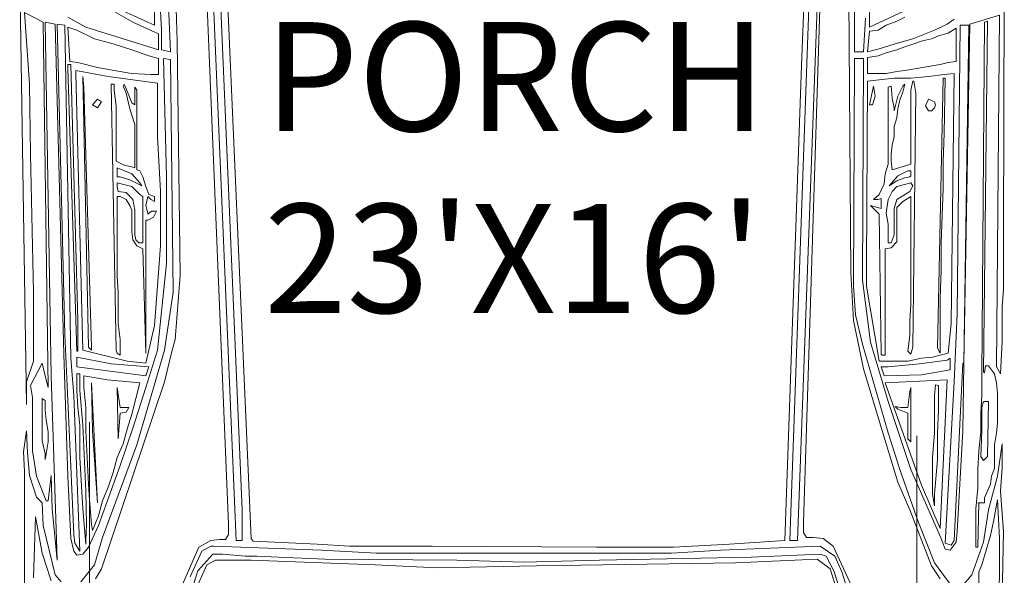
# Model space of a CAD drawing. Units: inches. Extents: x -9 to 646, y -802 to 47.
# Tile 5 of 17: x 432 to 486, y -633 to -602. Entities that reach past the tile are written whole.
import ezdxf

# ---------------------------------------------------------------- set-up
doc = ezdxf.new("R2010")
doc.units = ezdxf.units.IN
doc.header["$MEASUREMENT"] = 0
doc.layers.add('A-AREA-IDEN', color=7, linetype='Continuous', lineweight=18)
doc.layers.add('A-SITE-VEHI', color=8, linetype='Continuous', lineweight=9)
doc.styles.get("Standard").update_dxf_attribs({"font": 'arial.ttf'})

msp = doc.modelspace()

# ---------------------------------------------------------------- linework, layer by layer
at = {"layer": 'A-SITE-VEHI'}
for p, q in [((439.87, -602.535), (439.275, -591.315)), ((439.87, -591.424), (440.358, -603.727)), ((440.467, -594.892), (440.738, -603.132)), ((475.643, -597.277), (474.451, -630.612)), ((478.894, -596.79), (478.841, -602.373)), ((475.102, -604.487), (475.372, -597.821)), ((478.028, -603.727), (478.028, -597.765)), ((443.394, -598.092), (444.801, -630.503)), ((474.884, -630.612), (476.076, -598.254)), ((432.065, -599.608), (432.445, -623.132)), ((486.213, -613.808), (486.266, -599.77)), ((438.298, -602.102), (434.721, -600.041)), ((443.556, -629.744), (442.363, -600.53)), ((475.208, -629.635), (476.13, -600.476)), ((477.702, -600.312), (477.811, -615.869)), ((444.315, -628.931), (443.123, -600.909)), ((432.607, -605.517), (432.336, -601.56)), ((432.336, -601.56), (433.366, -602.102)), ((437.214, -601.234), (439.49, -602.264)), ((439.49, -602.264), (439.49, -601.398)), ((442.743, -601.505), (443.989, -630.612)), ((478.841, -602.373), (481.279, -601.234)), ((433.366, -602.102), (433.637, -622.21)), ((433.799, -621.56), (433.475, -602.102)), ((433.475, -602.102), (434.017, -602.211)), ((434.721, -601.831), (435.698, -602.373)), ((439.708, -602.752), (438.298, -602.102)), ((478.623, -601.884), (478.514, -603.727)), ((479.762, -602.264), (480.357, -602.048)), ((480.357, -602.048), (480.793, -601.831)), ((483.502, -601.94), (483.122, -602.211)), ((484.37, -602.211), (485.995, -601.722)), ((485.182, -602.102), (485.02, -621.56)), ((485.127, -621.342), (485.345, -602.048)), ((485.345, -602.048), (485.182, -602.102)), ((485.995, -601.722), (485.833, -621.071)), ((434.017, -602.211), (434.503, -620.367)), ((434.558, -602.264), (434.125, -602.211)), ((434.125, -602.211), (434.558, -619.284)), ((434.883, -620.585), (434.558, -602.264)), ((435.209, -602.535), (434.721, -602.373)), ((434.721, -602.373), (434.829, -604.269)), ((436.184, -603.023), (435.209, -602.535)), ((435.698, -602.373), (439.708, -603.618)), ((439.87, -603.618), (439.87, -602.535)), ((478.732, -603.727), (478.841, -602.59)), ((478.841, -602.59), (479.329, -602.535)), ((479.329, -602.535), (479.762, -602.264)), ((482.418, -602.535), (481.226, -603.023)), ((483.122, -602.211), (482.418, -602.535)), ((483.177, -602.697), (482.636, -602.861)), ((483.61, -602.426), (483.177, -602.697)), ((483.61, -604.269), (483.61, -602.426)), ((483.664, -618.145), (483.828, -602.264)), ((483.828, -602.264), (484.314, -602.264)), ((484.043, -620.856), (484.37, -602.211)), ((484.314, -602.264), (484.043, -620.856)), ((437.214, -603.294), (436.184, -603.023)), ((439.708, -603.618), (439.708, -602.752)), ((440.738, -603.132), (440.9, -616.031)), ((481.226, -603.023), (480.251, -603.294)), ((481.767, -603.132), (481.279, -603.294)), ((482.256, -603.023), (481.767, -603.132)), ((482.636, -602.861), (482.256, -603.023)), ((438.244, -603.618), (437.214, -603.294)), ((439.166, -603.945), (438.244, -603.618)), ((440.358, -603.727), (439.87, -603.618)), ((478.514, -603.727), (478.028, -603.727)), ((479.383, -603.565), (478.732, -603.727)), ((479.762, -603.783), (479.329, -603.945)), ((480.251, -603.294), (479.383, -603.565)), ((480.357, -603.618), (479.762, -603.783)), ((480.793, -603.456), (480.357, -603.618)), ((481.279, -603.294), (480.793, -603.456)), ((434.829, -604.269), (435.262, -604.324)), ((435.262, -604.324), (436.346, -604.595)), ((439.708, -604.107), (439.166, -603.945)), ((439.708, -604.975), (439.708, -604.107)), ((440.141, -610.611), (439.979, -604.107)), ((439.979, -604.107), (440.358, -604.162)), ((440.358, -604.162), (440.52, -616.952)), ((477.973, -616.628), (478.028, -604.107)), ((478.028, -604.107), (478.514, -604.107)), ((478.514, -604.107), (478.461, -616.302)), ((479.329, -603.945), (478.732, -604.054)), ((478.732, -604.054), (478.732, -604.92)), ((482.742, -604.433), (483.177, -604.324)), ((483.177, -604.324), (483.61, -604.269)), ((434.883, -604.433), (434.721, -604.433)), ((434.721, -604.433), (434.721, -604.649)), ((434.721, -604.649), (435.209, -620.205)), ((435.262, -618.524), (434.883, -604.433)), ((436.943, -605.082), (435.154, -604.757)), ((435.154, -604.757), (435.154, -604.92)), ((436.346, -604.595), (437.267, -604.757)), ((437.267, -604.757), (438.244, -604.92)), ((474.18, -630.612), (475.102, -604.487)), ((479.762, -604.92), (480.357, -604.811)), ((480.357, -604.811), (480.793, -604.757)), ((480.793, -604.757), (482.742, -604.433)), ((435.154, -604.92), (435.533, -620.15)), ((435.589, -605.679), (435.533, -605.082)), ((435.533, -605.082), (435.86, -619.987)), ((439.652, -605.461), (436.943, -605.082)), ((438.244, -604.92), (439.275, -604.975)), ((439.275, -604.975), (439.708, -604.975)), ((478.732, -605.355), (478.679, -615.544)), ((478.732, -604.92), (479.762, -604.92)), ((479.221, -605.299), (478.732, -605.355)), ((480.195, -605.19), (479.221, -605.299)), ((481.117, -605.19), (480.195, -605.19)), ((482.092, -605.082), (481.117, -605.19)), ((481.226, -605.355), (481.117, -605.841)), ((481.279, -605.355), (481.226, -605.355)), ((481.388, -606.003), (481.279, -605.355)), ((482.96, -604.975), (482.092, -605.082)), ((482.906, -605.19), (482.742, -613.051)), ((483.013, -605.19), (482.906, -605.19)), ((483.502, -604.92), (482.96, -604.975)), ((482.96, -608.226), (483.013, -605.19)), ((483.339, -618.686), (483.502, -604.92)), ((432.662, -609.365), (432.607, -605.517)), ((436.022, -619.987), (435.589, -605.679)), ((437.267, -605.517), (437.105, -605.517)), ((437.105, -605.517), (437.376, -620.15)), ((437.267, -605.841), (437.267, -605.517)), ((437.376, -606.709), (437.267, -605.841)), ((437.811, -605.517), (437.756, -605.626)), ((437.756, -605.626), (437.918, -606.003)), ((438.082, -606.112), (437.811, -605.517)), ((438.515, -605.841), (438.407, -605.679)), ((438.407, -605.679), (438.407, -606.654)), ((438.515, -610.231), (438.515, -605.841)), ((439.652, -608.388), (439.652, -605.461)), ((479.058, -605.626), (478.841, -606.654)), ((479.165, -606.167), (479.058, -605.626)), ((480.033, -605.626), (479.871, -605.679)), ((479.871, -605.679), (479.871, -609.907)), ((480.087, -606.276), (480.033, -605.626)), ((480.684, -605.626), (480.413, -606.167)), ((480.522, -606.383), (480.684, -605.95)), ((480.684, -605.95), (480.793, -605.517)), ((480.793, -605.517), (480.684, -605.626)), ((481.117, -605.841), (481.117, -609.907)), ((436.346, -606.329), (436.075, -606.654)), ((436.564, -606.492), (436.346, -606.329)), ((436.346, -606.818), (436.564, -606.492)), ((437.918, -606.003), (438.136, -606.871)), ((438.244, -606.547), (438.082, -606.112)), ((479.003, -606.654), (479.058, -606.492)), ((479.058, -606.492), (479.165, -606.167)), ((480.195, -606.818), (480.087, -606.276)), ((480.413, -606.167), (480.195, -606.98)), ((480.413, -606.871), (480.522, -606.383)), ((481.226, -619.987), (481.388, -606.003)), ((482.092, -606.329), (481.93, -606.709)), ((482.418, -606.492), (482.092, -606.329)), ((482.471, -606.654), (482.418, -606.492)), ((436.075, -606.654), (436.346, -606.818)), ((437.376, -609.745), (437.376, -606.709)), ((438.136, -606.871), (438.407, -607.739)), ((438.407, -606.654), (438.244, -606.547)), ((478.841, -606.654), (479.003, -606.654)), ((480.195, -606.98), (480.195, -606.818)), ((480.357, -607.36), (480.413, -606.871)), ((481.93, -606.709), (482.092, -606.98)), ((482.092, -606.98), (482.256, -606.98)), ((482.256, -606.98), (482.418, -606.818)), ((482.418, -606.818), (482.471, -606.654)), ((480.195, -607.846), (480.357, -607.36)), ((438.407, -607.739), (438.407, -610.124)), ((480.195, -608.388), (480.195, -607.846)), ((439.816, -611.423), (439.652, -608.388)), ((480.087, -608.876), (480.195, -608.388)), ((482.906, -609.745), (482.96, -608.226)), ((480.033, -609.365), (480.087, -608.876)), ((432.824, -616.952), (432.662, -609.365)), ((437.811, -609.96), (437.376, -609.745)), ((480.033, -609.745), (480.033, -609.365)), ((480.087, -610.231), (480.033, -609.745)), ((482.906, -611.261), (482.906, -609.745)), ((438.244, -610.448), (437.432, -610.124)), ((437.432, -610.124), (437.432, -610.611)), ((438.244, -610.069), (437.811, -609.96)), ((438.407, -610.124), (438.244, -610.069)), ((438.677, -610.286), (438.515, -610.231)), ((438.84, -610.611), (438.677, -610.286)), ((479.871, -609.907), (479.707, -610.448)), ((481.117, -609.907), (480.087, -610.231)), ((480.955, -610.286), (480.413, -610.557)), ((481.117, -610.286), (480.955, -610.286)), ((481.117, -610.557), (481.117, -610.286)), ((437.432, -610.611), (437.594, -610.611)), ((437.594, -610.611), (438.136, -610.775)), ((438.136, -610.775), (438.786, -611.099)), ((438.677, -610.937), (438.244, -610.448)), ((439.004, -611.152), (438.84, -610.611)), ((440.141, -615.38), (440.141, -610.611)), ((479.707, -610.448), (479.654, -610.99)), ((480.413, -610.557), (479.924, -611.099)), ((479.924, -611.099), (480.357, -610.828)), ((480.357, -610.828), (480.793, -610.666)), ((480.793, -610.666), (481.064, -610.611)), ((481.064, -610.611), (481.117, -610.557)), ((438.244, -611.152), (437.432, -610.937)), ((437.432, -610.937), (437.432, -611.152)), ((437.432, -611.152), (437.485, -611.423)), ((438.677, -611.587), (438.244, -611.152)), ((438.786, -611.099), (438.677, -610.937)), ((439.166, -611.587), (439.004, -611.152)), ((479.654, -610.99), (479.383, -611.587)), ((480.357, -611.152), (480.087, -611.423)), ((481.117, -610.937), (480.357, -611.152)), ((481.064, -611.423), (481.226, -611.099)), ((481.226, -611.099), (481.117, -610.937)), ((482.798, -614.243), (482.906, -611.261)), ((437.432, -616.086), (437.432, -611.696)), ((437.432, -611.696), (437.594, -611.696)), ((437.485, -611.423), (437.918, -611.479)), ((437.594, -611.696), (437.918, -611.858)), ((437.918, -611.479), (438.298, -611.858)), ((437.918, -611.858), (438.136, -612.183)), ((438.298, -611.858), (438.407, -612.454)), ((438.84, -611.696), (438.677, -611.587)), ((438.84, -614.243), (438.84, -611.696)), ((439.004, -612.183), (439.11, -611.696)), ((439.11, -611.696), (439.275, -611.858)), ((439.49, -611.696), (439.166, -611.587)), ((439.275, -611.858), (439.49, -611.967)), ((439.49, -611.967), (439.49, -611.696)), ((439.816, -614.405), (439.816, -611.423)), ((479.383, -611.587), (479.058, -611.858)), ((479.058, -611.858), (479.329, -611.858)), ((479.329, -611.858), (479.491, -611.803)), ((479.491, -611.803), (479.491, -612.345)), ((479.871, -611.858), (479.762, -612.616)), ((480.087, -611.423), (479.871, -611.858)), ((480.195, -612.345), (480.357, -611.858)), ((480.357, -611.858), (481.064, -611.423)), ((480.684, -611.967), (481.117, -611.696)), ((481.117, -611.696), (481.117, -617.658)), ((438.136, -612.183), (438.244, -612.454)), ((438.244, -612.454), (438.244, -613.646)), ((438.407, -612.454), (438.407, -613.808)), ((439.11, -612.616), (439.004, -612.183)), ((479.491, -612.345), (478.894, -612.183)), ((478.894, -612.183), (479.383, -612.671)), ((480.195, -613.808), (480.195, -612.345)), ((480.357, -612.291), (480.684, -611.967)), ((480.357, -614.188), (480.357, -612.291)), ((439.004, -620.314), (439.004, -612.995)), ((439.004, -612.995), (439.11, -612.995)), ((439.328, -612.509), (439.11, -612.671)), ((439.11, -612.671), (439.11, -612.616)), ((439.11, -612.995), (439.437, -612.833)), ((439.599, -612.509), (439.328, -612.509)), ((439.437, -612.833), (439.599, -612.509)), ((479.383, -612.671), (479.491, -620.367)), ((479.762, -612.616), (479.871, -613.213)), ((479.871, -613.213), (479.871, -614.243)), ((482.742, -613.051), (482.58, -620.043)), ((438.244, -613.646), (438.298, -614.081)), ((438.298, -614.081), (438.515, -614.405)), ((438.407, -613.808), (438.46, -614.081)), ((438.46, -614.081), (438.624, -614.243)), ((480.033, -614.243), (480.195, -613.808)), ((486.213, -616.79), (486.213, -613.808)), ((438.515, -614.405), (438.84, -614.567)), ((438.624, -614.243), (438.84, -614.243)), ((438.84, -614.567), (439.004, -620.314)), ((439.49, -618.795), (439.816, -614.405)), ((479.707, -614.567), (480.033, -614.514)), ((479.707, -620.423), (479.707, -614.567)), ((479.871, -614.243), (480.033, -614.243)), ((480.033, -614.514), (480.357, -614.188)), ((482.798, -615.76), (482.798, -614.243)), ((439.652, -620.15), (440.141, -615.38)), ((478.679, -615.544), (478.679, -616.628)), ((437.485, -616.952), (437.432, -616.086)), ((440.9, -616.031), (440.629, -619.554)), ((477.811, -615.869), (477.973, -618.524)), ((482.742, -617.278), (482.798, -615.76)), ((478.081, -618.2), (477.973, -616.628)), ((478.461, -616.302), (478.894, -619.717)), ((478.679, -616.628), (479.383, -620.747)), ((486.157, -617.765), (486.213, -616.79)), ((432.824, -620.747), (432.824, -616.952)), ((437.485, -618.686), (437.485, -616.952)), ((440.52, -616.952), (440.032, -620.15)), ((482.742, -620.314), (482.742, -617.278)), ((481.117, -617.658), (481.064, -618.524)), ((486.157, -619.663), (486.157, -617.765)), ((478.461, -619.825), (478.081, -618.2)), ((483.502, -621.886), (483.664, -618.145)), ((435.262, -620.205), (435.262, -618.524)), ((437.594, -619.554), (437.485, -618.686)), ((439.004, -620.856), (439.49, -618.795)), ((477.973, -618.524), (478.514, -621.18)), ((481.064, -618.524), (481.064, -619.337)), ((483.177, -620.314), (483.339, -618.686)), ((434.558, -619.284), (434.883, -626.547)), ((481.064, -619.337), (480.955, -620.205)), ((435.86, -619.987), (436.022, -620.15)), ((436.022, -620.15), (436.022, -619.987)), ((437.594, -620.423), (437.594, -619.554)), ((440.629, -619.554), (440.467, -620.15)), ((479.871, -624.704), (478.461, -619.825)), ((478.894, -619.717), (479.871, -622.97)), ((481.117, -620.367), (481.226, -619.987)), ((482.58, -620.043), (482.742, -620.314)), ((486.048, -621.451), (486.157, -619.663)), ((434.503, -620.367), (434.721, -627.088)), ((435.047, -622.643), (434.883, -620.585)), ((435.209, -620.205), (435.262, -620.205)), ((437.105, -620.909), (435.209, -620.529)), ((435.209, -620.529), (435.209, -621.071)), ((435.533, -620.15), (437.974, -620.747)), ((437.376, -620.15), (437.432, -620.314)), ((437.432, -620.314), (437.594, -620.423)), ((440.032, -620.15), (438.515, -625.354)), ((439.004, -622.21), (439.652, -620.15)), ((440.467, -620.15), (440.032, -621.886)), ((479.491, -620.367), (479.545, -620.423)), ((479.545, -620.423), (479.707, -620.423)), ((480.955, -620.205), (481.117, -620.367)), ((480.955, -620.747), (481.714, -620.585)), ((481.714, -620.585), (482.309, -620.529)), ((482.309, -620.529), (482.742, -620.423)), ((482.742, -620.423), (483.177, -620.314)), ((483.284, -620.585), (483.122, -620.694)), ((483.284, -621.235), (483.284, -620.585)), ((432.445, -621.886), (432.824, -620.747)), ((433.311, -620.856), (432.662, -622.101)), ((433.475, -621.56), (433.311, -620.856)), ((435.209, -621.071), (439.004, -621.56)), ((439.166, -621.071), (437.105, -620.909)), ((437.974, -620.747), (439.004, -620.856)), ((439.004, -621.56), (439.166, -621.071)), ((479.383, -620.747), (480.955, -620.747)), ((479.871, -621.071), (479.491, -621.071)), ((479.491, -621.071), (479.654, -621.56)), ((481.605, -620.909), (479.871, -621.071)), ((483.122, -620.694), (481.605, -620.909)), ((483.99, -620.856), (483.502, -630.612)), ((484.043, -620.856), (483.99, -620.856)), ((483.99, -624.595), (484.043, -620.909)), ((484.043, -620.909), (484.043, -620.856)), ((485.236, -621.018), (485.182, -621.397)), ((485.398, -621.018), (485.236, -621.018)), ((485.724, -621.451), (485.398, -621.018)), ((485.833, -621.071), (486.048, -621.451)), ((433.637, -622.21), (433.475, -621.56)), ((434.125, -631.696), (433.799, -621.56)), ((435.371, -621.451), (435.209, -621.451)), ((435.209, -621.451), (435.209, -622.372)), ((435.371, -622.372), (435.371, -621.451)), ((436.89, -621.777), (435.589, -621.56)), ((435.589, -621.56), (435.589, -622.21)), ((478.514, -621.18), (479.762, -625.299)), ((479.654, -621.56), (481.714, -621.506)), ((481.714, -621.506), (483.284, -621.235)), ((485.02, -621.56), (485.02, -622.643)), ((485.182, -621.397), (485.127, -621.342)), ((485.833, -621.939), (485.724, -621.451)), ((432.445, -623.132), (432.445, -621.886)), ((432.662, -622.101), (432.769, -622.752)), ((435.589, -622.21), (435.698, -623.294)), ((436.346, -628.552), (436.022, -621.939)), ((436.022, -621.939), (436.075, -624.595)), ((440.032, -621.886), (436.564, -632.182)), ((438.677, -621.939), (436.89, -621.777)), ((437.594, -623.294), (437.432, -622.21)), ((437.432, -622.21), (437.485, -625.028)), ((438.298, -624.433), (439.004, -622.21)), ((438.46, -622.807), (438.677, -621.939)), ((483.122, -621.777), (479.707, -621.939)), ((479.707, -621.939), (481.714, -627.577)), ((481.117, -622.21), (481.064, -622.428)), ((481.117, -625.192), (481.117, -622.21)), ((482.471, -622.048), (482.418, -622.643)), ((482.636, -622.101), (482.471, -622.048)), ((482.636, -623.456), (482.636, -622.101)), ((482.742, -629.962), (483.122, -621.777)), ((483.013, -630.774), (483.502, -621.886)), ((485.886, -622.536), (485.833, -621.939)), ((432.769, -622.752), (432.769, -625.678)), ((435.371, -631.207), (435.047, -622.643)), ((435.209, -622.372), (435.262, -623.294)), ((435.533, -624.271), (435.371, -622.372)), ((481.064, -622.428), (480.955, -623.294)), ((482.418, -622.643), (482.418, -624.704)), ((485.02, -622.643), (484.965, -623.62)), ((485.886, -624.162), (485.886, -622.536)), ((433.475, -622.914), (433.311, -622.807)), ((433.311, -622.807), (433.311, -625.137)), ((433.475, -623.456), (433.475, -622.914)), ((435.262, -623.294), (435.371, -624.271)), ((435.698, -623.294), (435.698, -624.595)), ((438.082, -623.294), (437.594, -623.294)), ((437.918, -623.565), (438.082, -623.294)), ((438.244, -623.673), (438.46, -622.807)), ((479.871, -622.97), (481.117, -626.709)), ((480.575, -623.294), (480.251, -623.24)), ((480.251, -623.24), (480.413, -623.403)), ((480.955, -623.294), (480.575, -623.294)), ((485.127, -622.97), (485.02, -623.294)), ((485.02, -623.294), (485.02, -624.595)), ((485.398, -622.97), (485.127, -622.97)), ((485.345, -626.005), (485.398, -622.97)), ((433.528, -624), (433.475, -623.456)), ((437.485, -625.028), (437.594, -623.62)), ((437.594, -623.62), (437.918, -623.565)), ((437.974, -624.486), (438.244, -623.673)), ((480.413, -623.403), (480.955, -623.62)), ((480.955, -623.62), (480.955, -625.028)), ((482.58, -624.704), (482.636, -623.456)), ((484.965, -623.62), (484.965, -624.648)), ((433.637, -624.648), (433.528, -624)), ((435.371, -624.271), (435.371, -626.058)), ((435.698, -627.901), (435.533, -624.271)), ((435.913, -624.106), (435.913, -643.944)), ((485.833, -624.704), (485.886, -624.162)), ((432.445, -624.595), (432.283, -625.734)), ((432.498, -625.787), (432.445, -624.595)), ((433.637, -625.192), (433.637, -624.648)), ((435.698, -624.595), (435.86, -627.521)), ((436.075, -624.595), (436.346, -628.552)), ((437.594, -626.491), (438.298, -624.433)), ((437.756, -625.299), (437.974, -624.486)), ((480.522, -626.709), (479.871, -624.704)), ((481.443, -624.866), (481.443, -644.812)), ((482.418, -624.704), (482.309, -626.058)), ((482.58, -626.167), (482.58, -624.704)), ((483.664, -630.124), (483.99, -624.595)), ((484.965, -624.648), (484.856, -625.678)), ((485.02, -624.595), (484.965, -626.005)), ((485.724, -625.354), (485.833, -624.704)), ((433.311, -625.137), (433.475, -625.843)), ((433.528, -625.843), (433.637, -625.192)), ((438.515, -625.354), (436.617, -630.448)), ((437.432, -626.058), (437.756, -625.299)), ((479.762, -625.299), (480.413, -627.413)), ((480.955, -625.028), (481.117, -625.192)), ((485.724, -626.655), (485.724, -625.354)), ((486.157, -625.299), (485.886, -627.088)), ((486.157, -626.6), (486.157, -625.299)), ((432.283, -625.734), (432.336, -626.818)), ((432.607, -627.035), (432.498, -625.787)), ((432.769, -625.678), (432.986, -627.088)), ((433.475, -626.167), (433.528, -625.843)), ((433.475, -625.843), (433.475, -626.167)), ((484.856, -625.678), (484.803, -626.709)), ((484.965, -626.005), (485.127, -626.22)), ((485.127, -626.22), (485.345, -626.005)), ((434.883, -626.547), (435.047, -630.286)), ((435.371, -626.058), (435.533, -628.876)), ((436.401, -629.797), (437.594, -626.491)), ((437.214, -626.871), (437.432, -626.058)), ((482.309, -626.058), (482.309, -628.063)), ((482.418, -628.063), (482.58, -626.167)), ((432.336, -626.818), (432.336, -636.303)), ((432.986, -628.228), (432.607, -627.035)), ((432.986, -627.088), (433.528, -628.443)), ((433.637, -628.443), (433.799, -627.035)), ((433.799, -627.035), (433.855, -628.876)), ((434.721, -627.088), (434.883, -630.503)), ((436.943, -627.684), (437.214, -626.871)), ((481.55, -629.635), (480.522, -626.709)), ((481.117, -626.709), (482.798, -630.503)), ((484.803, -626.709), (484.803, -627.739)), ((485.886, -627.088), (485.398, -628.931)), ((485.507, -627.521), (485.562, -627.088)), ((485.562, -627.088), (485.724, -626.655)), ((486.048, -627.901), (486.157, -626.6)), ((435.86, -627.521), (435.913, -628.39)), ((480.413, -627.413), (481.064, -628.931)), ((481.714, -627.577), (482.742, -629.962)), ((485.182, -628.281), (485.507, -627.521)), ((435.751, -629.744), (435.698, -627.901)), ((436.617, -628.443), (436.943, -627.684)), ((482.309, -628.063), (482.418, -628.714)), ((482.418, -628.714), (482.418, -628.063)), ((484.803, -627.739), (484.694, -628.876)), ((486.213, -630.124), (486.048, -627.901)), ((433.311, -628.552), (432.986, -628.228)), ((433.366, -629.797), (433.311, -628.552)), ((433.528, -628.443), (433.637, -628.443)), ((435.913, -628.39), (436.022, -629.744)), ((436.401, -629.256), (436.617, -628.443)), ((484.803, -630.99), (484.856, -628.552)), ((484.803, -628.552), (485.182, -628.552)), ((485.182, -628.552), (485.182, -628.281)), ((485.671, -629.582), (485.886, -628.39)), ((485.886, -628.39), (485.995, -630.503)), ((433.855, -628.876), (434.125, -631.696)), ((435.533, -628.876), (435.698, -630.828)), ((436.075, -630.068), (436.401, -629.256)), ((444.315, -630.612), (444.315, -628.931)), ((481.064, -628.931), (482.256, -632.02)), ((484.694, -628.876), (484.694, -630.99)), ((485.398, -628.931), (485.127, -630.719)), ((432.933, -629.311), (432.824, -632.671)), ((433.149, -630.503), (432.933, -629.311)), ((434.017, -632.509), (433.366, -629.797)), ((435.698, -630.612), (435.751, -629.744)), ((435.86, -630.99), (436.401, -629.797)), ((436.022, -629.744), (436.075, -630.068)), ((443.556, -630.286), (443.556, -629.744)), ((475.208, -630.177), (475.208, -629.635)), ((482.418, -631.858), (481.55, -629.635)), ((485.507, -630.341), (485.671, -629.582)), ((435.047, -630.286), (435.1, -630.774)), ((443.394, -630.557), (443.556, -630.286)), ((475.372, -630.448), (475.208, -630.177)), ((483.61, -630.719), (483.664, -630.124)), ((485.02, -631.967), (485.507, -630.341)), ((485.995, -640.855), (486.213, -630.124)), ((433.311, -631.316), (433.149, -630.503)), ((434.883, -630.503), (435.047, -631.207)), ((435.1, -630.774), (435.371, -631.207)), ((435.698, -630.828), (435.698, -630.612)), ((436.617, -630.448), (436.184, -631.967)), ((441.93, -630.99), (442.581, -630.612)), ((442.581, -630.612), (443.067, -630.557)), ((443.067, -630.557), (443.394, -630.557)), ((443.989, -630.612), (444.315, -630.612)), ((444.801, -630.503), (444.91, -630.666)), ((444.91, -630.666), (448.434, -630.828)), ((448.434, -630.828), (450.222, -630.936)), ((468.054, -630.99), (471.145, -630.828)), ((471.145, -630.828), (474.18, -630.612)), ((474.451, -630.612), (474.884, -630.612)), ((475.752, -630.448), (475.372, -630.448)), ((476.294, -630.503), (475.752, -630.448)), ((476.836, -630.936), (476.294, -630.503)), ((482.798, -630.503), (483.013, -631.099)), ((483.339, -630.883), (483.013, -630.774)), ((483.284, -631.154), (483.61, -630.719)), ((483.502, -630.612), (483.339, -630.883)), ((485.127, -630.719), (484.479, -632.509)), ((485.995, -630.503), (485.995, -632.509)), ((433.799, -632.833), (433.311, -631.316)), ((435.047, -631.207), (435.209, -631.425)), ((435.209, -631.425), (435.533, -631.37)), ((435.533, -631.37), (435.86, -630.99)), ((440.953, -633.212), (441.93, -630.99)), ((442.092, -631.207), (441.442, -632.617)), ((442.688, -631.37), (441.875, -632.291)), ((442.581, -630.936), (442.092, -631.207)), ((442.743, -630.936), (442.581, -630.936)), ((443.232, -631.37), (442.688, -631.37)), ((448.705, -631.154), (442.743, -630.936)), ((444.477, -631.478), (443.232, -631.37)), ((451.685, -631.316), (448.705, -631.154)), ((450.222, -630.936), (454.776, -630.936)), ((467.945, -631.316), (451.685, -631.316)), ((454.776, -630.936), (463.826, -630.99)), ((463.826, -630.99), (468.054, -630.99)), ((470.656, -631.154), (467.945, -631.316)), ((476.13, -630.936), (470.656, -631.154)), ((476.13, -631.37), (472.337, -631.534)), ((476.945, -631.478), (476.13, -630.936)), ((476.456, -631.478), (476.13, -631.37)), ((477.864, -633.159), (476.836, -630.936)), ((483.013, -631.099), (483.284, -631.154)), ((484.694, -630.99), (484.803, -630.99)), ((436.184, -631.967), (435.425, -632.888)), ((442.363, -631.967), (441.766, -633.321)), ((442.852, -631.696), (442.363, -631.967)), ((444.801, -631.696), (442.852, -631.696)), ((445.128, -631.478), (444.477, -631.478)), ((451.632, -631.967), (444.801, -631.696)), ((446.32, -631.534), (445.128, -631.478)), ((448.867, -631.64), (446.32, -631.534)), ((456.13, -631.696), (448.867, -631.64)), ((455.047, -632.129), (451.632, -631.967)), ((459.816, -631.805), (456.13, -631.696)), ((463.99, -631.696), (459.816, -631.805)), ((471.469, -631.858), (460.52, -632.02)), ((472.337, -631.534), (463.99, -631.696)), ((475.968, -631.64), (471.469, -631.858)), ((476.672, -632.182), (475.968, -631.64)), ((476.889, -632.291), (476.456, -631.478)), ((477.322, -632.346), (476.945, -631.478)), ((483.339, -633.104), (482.418, -631.858)), ((484.856, -632.346), (485.02, -631.967)), ((434.341, -632.888), (434.017, -632.509)), ((436.564, -632.182), (436.239, -632.726)), ((441.875, -632.291), (441.062, -634.785)), ((460.52, -632.02), (455.047, -632.129)), ((477.16, -633.701), (476.672, -632.182)), ((477.16, -633.159), (476.889, -632.291)), ((478.137, -634.947), (477.322, -632.346)), ((482.256, -632.02), (482.742, -632.726)), ((484.479, -632.509), (483.935, -633.159)), ((484.856, -633.159), (484.856, -632.346)), ((485.995, -632.509), (485.886, -636.574))]:
    msp.add_line(p, q, dxfattribs=at)

# ---------------------------------------------------------------- texts
at = {"layer": 'A-AREA-IDEN', "insert": (445.524, -602.097), "char_height": 6, "attachment_point": 1}
msp.add_mtext("PORCH\\P23'X16'", dxfattribs=at)

doc.saveas('drawing.dxf')
